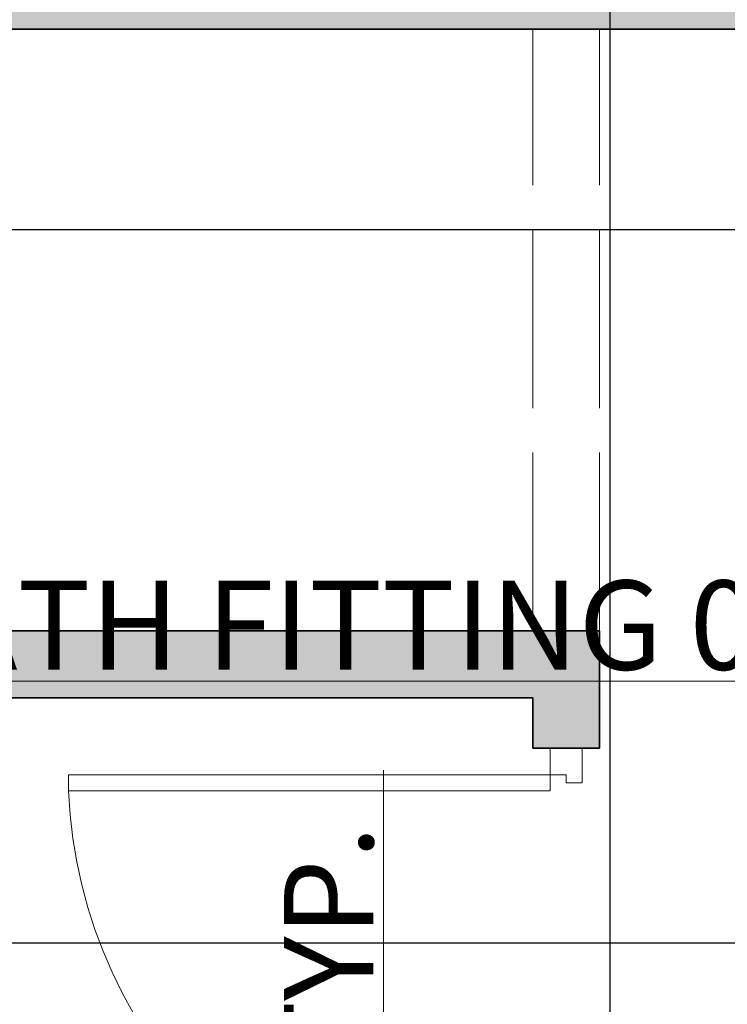
# Model space of a CAD drawing. Units: inches. Extents: x 2696 to 3240, y 1564 to 2310.
# Tile 50 of 76: x 2802 to 2850, y 2071 to 2137. Entities that reach past the tile are written whole.
import ezdxf

# ---------------------------------------------------------------- set-up
doc = ezdxf.new("R2010")
doc.units = ezdxf.units.IN
doc.linetypes.add('ACAD_ISO02W100', pattern=[15, 12, -3])
for name, color, linetype, lineweight in [('A-ANNO-DIMS', 3, 'Continuous', 18), ('A-DOOR', 4, 'Continuous', 18), ('A-WALL', 7, 'Continuous', 35), ('A-WALL-OVHD', 7, 'ACAD_ISO02W100', 18), ('A-WALL-PATT', 9, 'Continuous', 13)]:
    doc.layers.add(name, color=color, linetype=linetype, lineweight=lineweight)
doc.styles.add('TIMES NEW', font='times.ttf')
doc.dimstyles.new('Siddhuu', dxfattribs={"dimtxt": 6, "dimasz": 2.5, "dimexe": 1.25, "dimexo": 0.625, "dimtad": 1, "dimdec": 1, "dimlunit": 4, "dimtxsty": 'TIMES NEW', "dimcen": 2.5, "dimclrd": 256, "dimclre": 1, "dimclrt": 7, "dimadec": 0, "dimazin": 0, "dimtfac": 1, "dimtdec": 1, "dimtmove": 0, "dimatfit": 3, "dimfxl": 1, "dimtolj": 1, "dimlwd": -1, "dimarcsym": 0})

# ---------------------------------------------------------------- blocks, each defined once
blk = doc.blocks.new('DR_D01')
for p, q in [((-0.45, 0.93), (-0.42, 0.93)), ((-0.45, 0.03), (-0.45, 0.93)), ((-0.42, 0.03), (-0.42, 0.93)), ((-0.5, 0.03), (-0.42, 0.03)), ((-0.5, 0.03), (-0.5, -0.03)), ((-0.45, 0.03), (-0.45, 0)), ((0.45, 0.03), (0.45, 0)), ((0.5, 0.03), (0.45, 0.03)), ((0.5, -0.03), (0.5, 0.03)), ((-0.45, 0), (-0.435, 0)), ((-0.435, 0), (-0.435, -0.03)), ((0.435, 0), (0.435, -0.03)), ((0.45, 0), (0.435, 0)), ((-0.435, -0.03), (-0.5, -0.03)), ((0.435, -0.03), (0.5, -0.03))]:
    blk.add_line(p, q)
blk.add_arc((-0.4602, 0.0206), 0.9103, 0.5915, 87.4664)
blk = doc.blocks.new('*D40')
at = {"layer": 'A-ANNO-DIMS', "color": 1, "lineweight": -2, "transparency": 16777216}
for p, q in [((2777.266, 2091.826), (2777.266, 2093.576)), ((2784.764, 2091.826), (2784.764, 2093.576))]:
    blk.add_line(p, q, dxfattribs=at)
at = {"layer": 'A-ANNO-DIMS', "transparency": 16777216}
for p, q in [((2779.766, 2092.326), (2782.264, 2092.326)), ((2784.764, 2092.326), (2902.458, 2092.326))]:
    blk.add_line(p, q, dxfattribs=at)
for points in [[(2779.766, 2092.742), (2779.766, 2091.909), (2777.266, 2092.326)], [(2782.264, 2092.742), (2782.264, 2091.909), (2784.764, 2092.326)]]:
    blk.add_solid(points, dxfattribs=at)
at = {"layer": 'Defpoints', "color": 0, "transparency": 16777216}
for p in [(2784.764, 2092.326), (2777.266, 2091.201), (2784.764, 2091.201)]:
    blk.add_point(p, dxfattribs=at)
at = {"layer": 'A-ANNO-DIMS', "color": 7, "transparency": 16777216, "insert": (2844.861, 2096.094), "char_height": 6, "attachment_point": 5, "style": 'TIMES NEW'}
blk.add_mtext('\\A1;BATH FITTING 0\'-7 1/2" TYP.', dxfattribs=at)
blk = doc.blocks.new('*D44')
at = {"layer": 'A-ANNO-DIMS', "transparency": 16777216}
for p, q in [((2826.678, 1989.067), (2826.678, 2086.33)), ((2826.678, 1944.454), (2826.678, 1986.567))]:
    blk.add_line(p, q, dxfattribs=at)
at = {"layer": 'A-ANNO-DIMS', "color": 1, "lineweight": -2, "transparency": 16777216}
for p, q in [((2820.236, 1989.067), (2827.928, 1989.067)), ((2820.236, 1941.954), (2827.928, 1941.954))]:
    blk.add_line(p, q, dxfattribs=at)
at = {"layer": 'A-ANNO-DIMS', "transparency": 16777216}
for points in [[(2826.261, 1986.567), (2827.094, 1986.567), (2826.678, 1989.067)], [(2826.261, 1944.454), (2827.094, 1944.454), (2826.678, 1941.954)]]:
    blk.add_solid(points, dxfattribs=at)
at = {"layer": 'Defpoints', "color": 0, "transparency": 16777216}
for p in [(2819.611, 1989.067), (2826.678, 1989.067), (2819.611, 1941.954)]:
    blk.add_point(p, dxfattribs=at)
at = {"layer": 'A-ANNO-DIMS', "color": 7, "transparency": 16777216, "insert": (2822.986, 2038.948), "char_height": 6, "attachment_point": 5, "rotation": 90, "style": 'TIMES NEW'}
blk.add_mtext('\\A1;DINING SET 3\'-11" TYP.', dxfattribs=at)
blk = doc.blocks.new('*D62')
at = {"layer": 'A-ANNO-DIMS', "color": 1, "lineweight": -2, "transparency": 16777216}
for p, q in [((2965.084, 2140.701), (2709.361, 2140.701)), ((2965.084, 2063.591), (2709.361, 2063.591))]:
    blk.add_line(p, q, dxfattribs=at)
at = {"layer": 'A-ANNO-DIMS', "transparency": 16777216}
blk.add_line((2710.611, 2066.091), (2710.611, 2138.201), dxfattribs=at)
for points in [[(2710.195, 2138.201), (2711.028, 2138.201), (2710.611, 2140.701)], [(2710.195, 2066.091), (2711.028, 2066.091), (2710.611, 2063.591)]]:
    blk.add_solid(points, dxfattribs=at)
at = {"layer": 'Defpoints', "color": 0, "transparency": 16777216}
for p in [(2710.611, 2140.701), (2965.709, 2140.701), (2965.709, 2063.591)]:
    blk.add_point(p, dxfattribs=at)
at = {"layer": 'A-ANNO-DIMS', "color": 7, "transparency": 16777216, "insert": (2706.934, 2102.146), "char_height": 6, "attachment_point": 5, "rotation": 90, "style": 'TIMES NEW'}
blk.add_mtext('\\A1;6\'-5"', dxfattribs=at)
blk = doc.blocks.new('*D64')
at = {"layer": 'A-ANNO-DIMS', "color": 1, "lineweight": -2, "transparency": 16777216}
for p, q in [((3073.084, 2206.701), (2709.361, 2206.701)), ((3068.584, 1989.201), (2709.361, 1989.201))]:
    blk.add_line(p, q, dxfattribs=at)
at = {"layer": 'A-ANNO-DIMS', "transparency": 16777216}
blk.add_line((2710.611, 1991.701), (2710.611, 2204.201), dxfattribs=at)
for points in [[(2710.195, 2204.201), (2711.028, 2204.201), (2710.611, 2206.701)], [(2710.195, 1991.701), (2711.028, 1991.701), (2710.611, 1989.201)]]:
    blk.add_solid(points, dxfattribs=at)
at = {"layer": 'Defpoints', "color": 0, "transparency": 16777216}
for p in [(2710.611, 2206.701), (3073.709, 2206.701), (3069.209, 1989.201)]:
    blk.add_point(p, dxfattribs=at)
at = {"layer": 'A-ANNO-DIMS', "color": 7, "transparency": 16777216, "insert": (2706.85, 2097.951), "char_height": 6, "attachment_point": 5, "rotation": 90, "style": 'TIMES NEW'}
blk.add_mtext('\\A1;18\'-1 1/2"', dxfattribs=at)
blk = doc.blocks.new('*D66')
at = {"layer": 'A-ANNO-DIMS', "color": 1, "lineweight": -2, "transparency": 16777216}
for p, q in [((3077.584, 2122.701), (2709.361, 2122.701)), ((3077.584, 2074.701), (2709.361, 2074.701))]:
    blk.add_line(p, q, dxfattribs=at)
at = {"layer": 'A-ANNO-DIMS', "transparency": 16777216}
blk.add_line((2710.611, 2077.201), (2710.611, 2120.201), dxfattribs=at)
for points in [[(2710.195, 2120.201), (2711.028, 2120.201), (2710.611, 2122.701)], [(2710.195, 2077.201), (2711.028, 2077.201), (2710.611, 2074.701)]]:
    blk.add_solid(points, dxfattribs=at)
at = {"layer": 'Defpoints', "color": 0, "transparency": 16777216}
for p in [(2710.611, 2122.701), (3078.209, 2122.701), (3078.209, 2074.701)]:
    blk.add_point(p, dxfattribs=at)
at = {"layer": 'A-ANNO-DIMS', "color": 7, "transparency": 16777216, "insert": (2706.934, 2098.701), "char_height": 6, "attachment_point": 5, "rotation": 90, "style": 'TIMES NEW'}
blk.add_mtext('\\A1;4\'-0"', dxfattribs=at)
blk = doc.blocks.new('*D69')
at = {"layer": 'A-ANNO-DIMS', "color": 1, "lineweight": -2, "transparency": 16777216}
for p, q in [((2841.889, 2261.576), (2841.889, 1568.951)), ((2905.91, 2261.576), (2905.91, 1568.951))]:
    blk.add_line(p, q, dxfattribs=at)
at = {"layer": 'A-ANNO-DIMS', "transparency": 16777216}
blk.add_line((2844.389, 1570.201), (2903.41, 1570.201), dxfattribs=at)
for points in [[(2844.389, 1570.618), (2844.389, 1569.784), (2841.889, 1570.201)], [(2903.41, 1570.618), (2903.41, 1569.784), (2905.91, 1570.201)]]:
    blk.add_solid(points, dxfattribs=at)
at = {"layer": 'Defpoints', "color": 0, "transparency": 16777216}
for p in [(2841.889, 2262.201), (2905.91, 2262.201), (2905.91, 1570.201)]:
    blk.add_point(p, dxfattribs=at)
at = {"layer": 'A-ANNO-DIMS', "color": 7, "transparency": 16777216, "insert": (2873.9, 1573.878), "char_height": 6, "attachment_point": 5, "style": 'TIMES NEW'}
blk.add_mtext('\\A1;5\'-4"', dxfattribs=at)

msp = doc.modelspace()

# ---------------------------------------------------------------- hatches: boundary and pattern name
at = {"layer": 'A-WALL-PATT', "transparency": 33554556}
h = msp.add_hatch(color=256, dxfattribs=at)
h.dxf.hatch_style = 1
h.paths.add_polyline_path([(2879.111, 2253.201), (2905.91, 2253.201), (2905.91, 2262.201), (2841.889, 2262.201), (2841.889, 2253.201), (2870.111, 2253.201), (2870.111, 2176.601), (2965.709, 2176.601), (2965.709, 2206.701), (2973.583, 2206.701), (2973.583, 2215.701), (2965.709, 2215.701), (2965.709, 2262.201), (2929.91, 2262.201), (2929.91, 2253.201), (2956.709, 2253.201), (2956.709, 2185.601), (2879.111, 2185.601)])
h.paths.add_polyline_path([(2782.834, 2262.201), (2745.611, 2262.201), (2745.611, 2228.729), (2754.611, 2228.729), (2754.611, 2253.201), (2782.834, 2253.201)])
h.paths.add_polyline_path([(2754.611, 2136.201), (2965.709, 2136.201), (2965.709, 2145.201), (2879.111, 2145.201), (2879.111, 2147.074), (2877.34, 2147.074), (2870.111, 2147.074), (2870.111, 2145.201), (2754.611, 2145.201), (2754.611, 2169.674), (2745.611, 2169.674), (2745.611, 2000.201), (2754.611, 2000.201), (2754.611, 2019.201), (2849.083, 2019.201), (2849.083, 2023.701), (2841.209, 2023.701), (2841.209, 2051.827), (2836.709, 2051.827), (2836.709, 2023.701), (2754.611, 2023.701), (2754.611, 2091.201), (2836.709, 2091.201), (2836.709, 2087.827), (2841.209, 2087.827), (2841.209, 2095.701), (2754.611, 2095.701)])
h.paths.add_polyline_path([(2965.709, 2136.201), (2956.709, 2136.201), (2956.709, 2023.701), (2885.083, 2023.701), (2885.083, 2019.201), (2956.709, 2019.201), (2956.709, 1950.575), (2965.709, 1950.575), (2965.709, 1980.201), (2973.583, 1980.201), (2973.583, 1989.201), (2965.709, 1989.201)])
h.paths.add_polyline_path([(2754.611, 1906.701), (2880.209, 1906.701), (2884.709, 1906.701), (2956.709, 1906.701), (2956.709, 1792.701), (2944.709, 1792.701), (2944.709, 1783.701), (2956.709, 1783.701), (2956.709, 1740.201), (2884.709, 1740.201), (2884.709, 1783.701), (2896.709, 1783.701), (2896.709, 1792.701), (2884.709, 1792.701), (2884.709, 1846.701), (2880.209, 1846.701), (2880.209, 1740.201), (2754.611, 1740.201), (2754.611, 1777.201), (2745.611, 1777.201), (2745.611, 1692.701), (2754.611, 1692.701), (2754.611, 1731.201), (2956.709, 1731.201), (2956.709, 1723.327), (2965.709, 1723.327), (2965.709, 1884.201), (2973.583, 1884.201), (2973.583, 1893.201), (2965.709, 1893.201), (2965.709, 1914.575), (2956.709, 1914.575), (2956.709, 1911.201), (2754.611, 1911.201), (2754.611, 1930.201), (2745.611, 1930.201), (2745.611, 1817.201), (2754.611, 1817.201), (2754.611, 1854.201), (2826.611, 1854.201), (2826.611, 1868.827), (2822.111, 1868.827), (2822.111, 1858.701), (2754.611, 1858.701)])
h.paths.add_polyline_path([(2965.709, 1656.201), (3008.237, 1656.201), (3008.237, 1665.201), (2965.709, 1665.201), (2965.709, 1693.327), (2956.709, 1693.327), (2956.709, 1686.201), (2934.583, 1686.201), (2934.583, 1681.701), (2956.709, 1681.701), (2956.709, 1614.201), (2896.709, 1614.201), (2896.709, 1681.701), (2904.583, 1681.701), (2904.583, 1686.201), (2892.209, 1686.201), (2892.209, 1614.201), (2858.41, 1614.201), (2858.41, 1605.201), (2965.709, 1605.201)])
h.paths.add_polyline_path([(2788.41, 1614.201), (2754.611, 1614.201), (2754.611, 1652.701), (2745.611, 1652.701), (2745.611, 1605.201), (2788.41, 1605.201)])
h.paths.add_polyline_path([(3199.611, 1633.048), (3190.611, 1633.048), (3190.611, 1614.201), (3082.611, 1614.201), (3082.611, 1665.201), (3070.237, 1665.201), (3070.237, 1656.201), (3078.111, 1656.201), (3078.111, 1605.201), (3199.611, 1605.201)])
h.paths.add_polyline_path([(3199.611, 1702.048), (3190.611, 1702.048), (3190.611, 1699.701), (3106.611, 1699.701), (3106.611, 1747.701), (3190.611, 1747.701), (3190.611, 1752.201), (3082.611, 1752.201), (3082.611, 1760.075), (3078.111, 1760.075), (3078.111, 1747.701), (3102.111, 1747.701), (3102.111, 1699.701), (3078.111, 1699.701), (3078.111, 1695.201), (3190.611, 1695.201), (3190.611, 1676.355), (3199.611, 1676.355)])
h.paths.add_polyline_path([(3199.611, 1783.201), (3190.611, 1783.201), (3190.611, 1745.355), (3199.611, 1745.355)])
h.paths.add_polyline_path([(3082.611, 1884.201), (3190.611, 1884.201), (3190.611, 1853.201), (3199.611, 1853.201), (3199.611, 1901.701), (3190.611, 1901.701), (3190.611, 1893.201), (3005.583, 1893.201), (3005.583, 1891.281), (3005.583, 1884.201), (3078.111, 1884.201), (3078.111, 1792.075), (3082.611, 1792.075)])
h.paths.add_polyline_path([(3199.611, 1994.701), (3190.611, 1994.701), (3190.611, 1989.201), (3073.709, 1989.201), (3073.709, 2034.201), (3069.209, 2034.201), (3069.209, 1989.201), (3005.583, 1989.201), (3005.583, 1980.201), (3190.611, 1980.201), (3190.611, 1971.701), (3199.611, 1971.701)])
h.paths.add_polyline_path([(3199.611, 2155.201), (3190.611, 2155.201), (3190.611, 2064.701), (3199.611, 2064.701)])
h.paths.add_polyline_path([(3190.611, 2074.701), (3106.611, 2074.701), (3106.611, 2122.701), (3190.611, 2122.701), (3190.611, 2127.201), (3082.709, 2127.201), (3082.709, 2135.075), (3073.709, 2135.075), (3073.709, 2122.701), (3102.111, 2122.701), (3102.111, 2074.701), (3069.209, 2074.701), (3069.209, 2070.201), (3190.611, 2070.201)])
h.paths.add_polyline_path([(3082.709, 2253.201), (3190.611, 2253.201), (3190.611, 2225.201), (3199.611, 2225.201), (3199.611, 2262.201), (3073.709, 2262.201), (3073.709, 2215.701), (3035.583, 2215.701), (3035.583, 2206.701), (3073.709, 2206.701), (3073.709, 2171.075), (3082.709, 2171.075)])

# ---------------------------------------------------------------- linework, layer by layer
at = {"layer": 'A-WALL'}
for p, q in [((2754.611, 2136.201), (2965.709, 2136.201)), ((2754.611, 2095.701), (2841.209, 2095.701)), ((2841.209, 2095.701), (2841.209, 2087.827)), ((2754.611, 2091.201), (2836.709, 2091.201)), ((2836.709, 2091.201), (2836.709, 2087.827)), ((2841.209, 2087.827), (2836.709, 2087.827))]:
    msp.add_line(p, q, dxfattribs=at)
at = {"layer": 'A-WALL-OVHD'}
for p, q in [((2836.709, 2095.701), (2836.709, 2136.201)), ((2841.209, 2095.701), (2841.209, 2136.201))]:
    msp.add_line(p, q, dxfattribs=at)

# ---------------------------------------------------------------- block references
at = {"layer": 'A-DOOR', "xscale": 36, "yscale": -36, "zscale": 36, "rotation": 270.0000000000007}
msp.add_blockref('DR_D01', (2838.959, 2069.827), dxfattribs=at)

# ---------------------------------------------------------------- dimensions: what is measured, and where the dimension line sits
at = {"layer": 'A-ANNO-DIMS'}
dim = msp.add_linear_dim(base=(2905.91, 1570.201), p1=(2841.889, 2262.201), p2=(2905.91, 2262.201), dimstyle='Siddhuu', override={"dimdec": 1, "dimlfac": 1, "dimrnd": 0, "dimzin": 1, "dimdsep": 46, "dimlunit": 4, "dimfrac": 2}, dxfattribs=at)
dim.commit()
dim.dimension.update_dxf_attribs({"geometry": '*D69', "text_midpoint": (2873.9, 1573.878)})
for base, p1, p2, picture, middle in [((2710.611, 2206.701), (3069.209, 1989.201), (3073.709, 2206.701), '*D64', (2706.85, 2097.951)), ((2710.611, 2140.701), (2965.709, 2063.591), (2965.709, 2140.701), '*D62', (2706.934, 2102.146)), ((2710.611, 2122.701), (3078.209, 2074.701), (3078.209, 2122.701), '*D66', (2706.934, 2098.701))]:
    dim = msp.add_linear_dim(base=base, p1=p1, p2=p2, angle=90, dimstyle='Siddhuu', override={"dimdec": 1, "dimlfac": 1, "dimrnd": 0, "dimzin": 1, "dimdsep": 46, "dimlunit": 4, "dimfrac": 2}, dxfattribs=at)
    dim.commit()
    dim.dimension.update_dxf_attribs({"geometry": picture, "text_midpoint": middle})
dim = msp.add_linear_dim(base=(2784.764, 2092.326), p1=(2777.266, 2091.201), p2=(2784.764, 2091.201), text='BATH FITTING <> TYP.', dimstyle='Siddhuu', override={"dimdec": 1, "dimlfac": 1, "dimrnd": 0, "dimzin": 1, "dimdsep": 46, "dimlunit": 4, "dimfrac": 2}, dxfattribs=at)
dim.commit()
dim.dimension.update_dxf_attribs({"geometry": '*D40', "text_midpoint": (2844.861, 2096.094)})
dim = msp.add_linear_dim(base=(2826.678, 1989.067), p1=(2819.611, 1941.954), p2=(2819.611, 1989.067), angle=90, text='DINING SET <> TYP.', dimstyle='Siddhuu', override={"dimdec": 1, "dimlfac": 1, "dimrnd": 0, "dimzin": 1, "dimdsep": 46, "dimlunit": 4, "dimfrac": 2}, dxfattribs=at)
dim.commit()
dim.dimension.update_dxf_attribs({"geometry": '*D44', "text_midpoint": (2822.986, 2038.948)})

doc.saveas('drawing.dxf')
